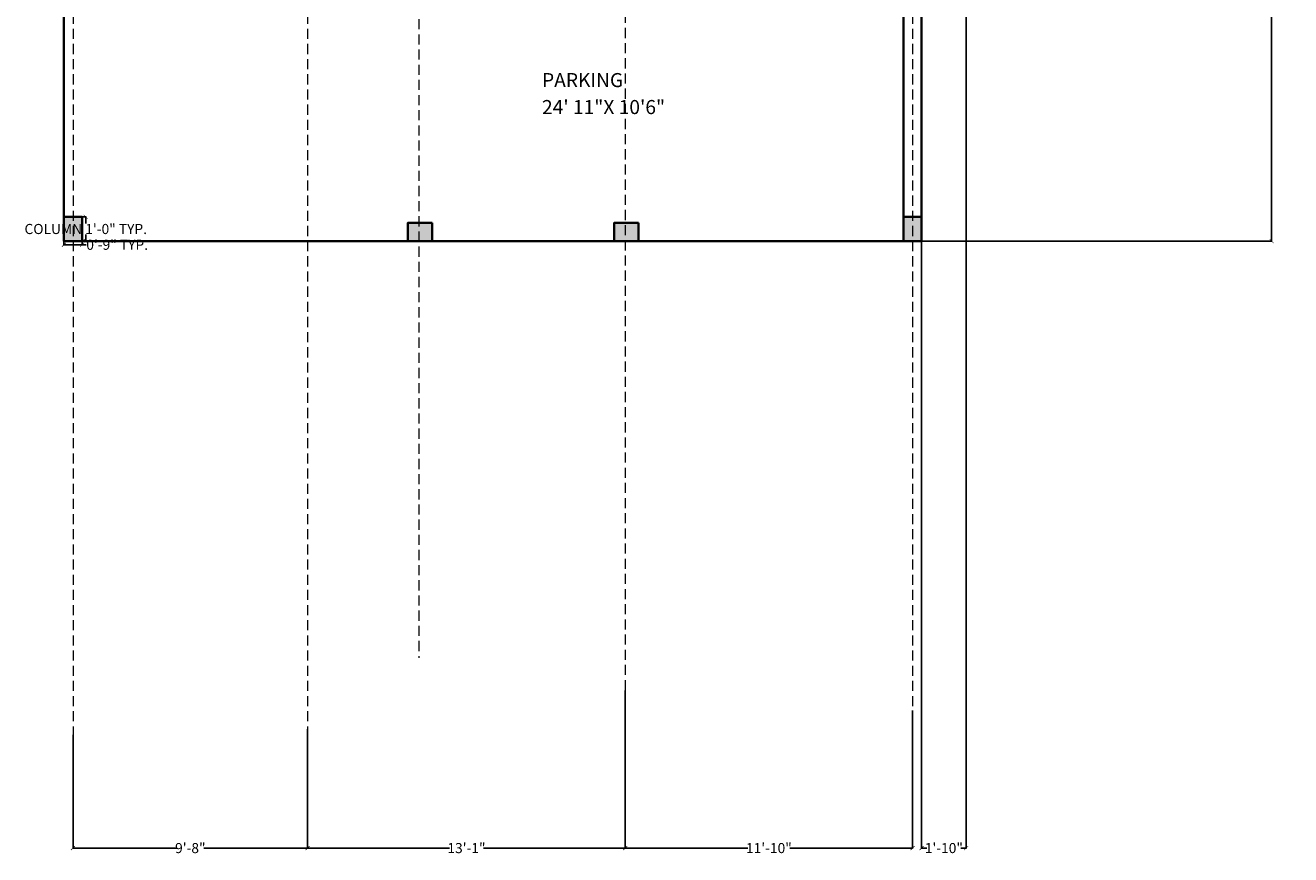
# Model space of a CAD drawing. Units: inches. Extents: x 782 to 2660, y -1008 to 166.
# Tile 1 of 12: x 964 to 1589, y -1008 to -598. Entities that reach past the tile are written whole.
import ezdxf

# ---------------------------------------------------------------- set-up
doc = ezdxf.new("R2010")
doc.units = ezdxf.units.IN
doc.header["$MEASUREMENT"] = 0
doc.linetypes.add('DASHED', pattern=[0.75, 0.5, -0.25])
for name, color, linetype, lineweight in [('A-ANNO-DIMS', 4, 'Continuous', 18), ('A-AREA-IDEN', 4, 'Continuous', 18), ('A-COLS', 7, 'Continuous', 35), ('A-GRID', 8, 'DASHED', 13), ('A-WALL', 7, 'Continuous', 35)]:
    doc.layers.add(name, color=color, linetype=linetype, lineweight=lineweight)
doc.styles.get("Standard").update_dxf_attribs({"font": 'arial.ttf'})
doc.dimstyles.get("Standard").update_dxf_attribs({"dimtxt": 5, "dimasz": 2, "dimexe": 0.18, "dimexo": 0.0625, "dimgap": 0.09, "dimtad": 0, "dimtih": 1, "dimtoh": 1, "dimdec": 0, "dimzin": 0, "dimdsep": 46, "dimlunit": 3, "dimtxsty": 'Standard', "dimblk": 'ARCHTICK', "dimcen": 0.09, "dimadec": 0, "dimazin": 0, "dimtfac": 1, "dimtdec": 0, "dimtofl": 0, "dimtmove": 0, "dimatfit": 3, "dimfxl": 1, "dimtolj": 1, "dimtzin": 0, "dimarcsym": 0})

# ---------------------------------------------------------------- blocks, each defined once
blk = doc.blocks.new('COL-9X12')
h = blk.add_hatch(color=256)
h.dxf.hatch_style = 1
h.paths.add_polyline_path([(9, 12), (0, 12), (0, 0), (9, 0)])
blk.add_lwpolyline([(0, 12), (9, 12), (9, 0), (0, 0)], close=True)
blk = doc.blocks.new('_ArchTick')
at = {"color": 0, "linetype": 'ByBlock', "const_width": 0.15}
blk.add_lwpolyline([(-0.5, -0.5), (0.5, 0.5)], dxfattribs=at)
blk = doc.blocks.new('*D25')
at = {"layer": 'A-ANNO-DIMS', "color": 0, "lineweight": -2, "transparency": 16777216}
for p, q in [((991.75, -692.99), (993.66, -692.99)), ((993.48, -692.99), (993.48, -696.32)), ((991.75, -704.99), (993.66, -704.99)), ((993.48, -704.99), (993.48, -701.67))]:
    blk.add_line(p, q, dxfattribs=at)
at = {"layer": 'Defpoints', "color": 0, "transparency": 16777216}
for p in [(991.68, -692.99), (993.48, -692.99), (991.68, -704.99)]:
    blk.add_point(p, dxfattribs=at)
at = {"layer": 'A-ANNO-DIMS', "color": 0, "lineweight": -2, "transparency": 16777216, "xscale": 2, "yscale": 2, "zscale": 2}
for p, rotation in [((993.48, -692.99), 90), ((993.48, -704.99), 270)]:
    blk.add_blockref('_ArchTick', p, dxfattribs=dict(at, rotation=rotation))
at = {"layer": 'A-ANNO-DIMS', "color": 0, "transparency": 16777216, "insert": (993.48, -698.99), "char_height": 5, "attachment_point": 5}
blk.add_mtext('\\A1;COLUMN 1\'-0" TYP.', dxfattribs=at)
blk = doc.blocks.new('*D26')
at = {"layer": 'A-ANNO-DIMS', "color": 0, "lineweight": -2, "transparency": 16777216}
for p, q in [((982.68, -705.06), (982.68, -706.97)), ((982.68, -706.79), (991.68, -706.79)), ((991.68, -705.06), (991.68, -706.97)), ((991.68, -706.79), (993.68, -706.79))]:
    blk.add_line(p, q, dxfattribs=at)
at = {"layer": 'Defpoints', "color": 0, "transparency": 16777216}
for p in [(982.68, -704.99), (991.68, -704.99), (991.68, -706.79)]:
    blk.add_point(p, dxfattribs=at)
at = {"layer": 'A-ANNO-DIMS', "color": 0, "lineweight": -2, "transparency": 16777216, "xscale": 2, "yscale": 2, "zscale": 2, "rotation": 180}
blk.add_blockref('_ArchTick', (982.68, -706.79), dxfattribs=at)
at = {"layer": 'A-ANNO-DIMS', "color": 0, "lineweight": -2, "transparency": 16777216, "xscale": 2, "yscale": 2, "zscale": 2}
blk.add_blockref('_ArchTick', (991.68, -706.79), dxfattribs=at)
at = {"layer": 'A-ANNO-DIMS', "color": 0, "transparency": 16777216, "insert": (1009.01, -706.79), "char_height": 5, "attachment_point": 5}
blk.add_mtext('\\A1;0\'-9" TYP.', dxfattribs=at)
blk = doc.blocks.new('*D51')
at = {"layer": 'A-ANNO-DIMS', "color": 0, "lineweight": -2, "transparency": 16777216}
for p, q in [((1406.75, 45.01), (1579.89, 45.01)), ((1579.71, 45.01), (1579.71, -327.35)), ((1579.71, -704.99), (1579.71, -332.64)), ((1406.75, -704.99), (1579.89, -704.99))]:
    blk.add_line(p, q, dxfattribs=at)
at = {"layer": 'Defpoints', "color": 0, "transparency": 16777216}
for p in [(1406.68, 45.01), (1579.71, 45.01), (1406.68, -704.99)]:
    blk.add_point(p, dxfattribs=at)
at = {"layer": 'A-ANNO-DIMS', "color": 0, "lineweight": -2, "transparency": 16777216, "xscale": 2, "yscale": 2, "zscale": 2}
for p, rotation in [((1579.71, 45.01), 90), ((1579.71, -704.99), 270)]:
    blk.add_blockref('_ArchTick', p, dxfattribs=dict(at, rotation=rotation))
at = {"layer": 'A-ANNO-DIMS', "color": 0, "transparency": 16777216, "insert": (1579.71, -329.99), "char_height": 5, "attachment_point": 5}
blk.add_mtext('\\A1;62\'-6"', dxfattribs=at)
blk = doc.blocks.new('*D53')
at = {"layer": 'A-ANNO-DIMS', "color": 0, "lineweight": -2, "transparency": 16777216}
for p, q in [((1406.68, -579.06), (1406.68, -1005.36)), ((1428.68, -579.06), (1428.68, -1005.36)), ((1406.68, -1005.18), (1409.24, -1005.18)), ((1428.68, -1005.18), (1426.13, -1005.18))]:
    blk.add_line(p, q, dxfattribs=at)
at = {"layer": 'Defpoints', "color": 0, "transparency": 16777216}
for p in [(1406.68, -578.99), (1428.68, -578.99), (1428.68, -1005.18)]:
    blk.add_point(p, dxfattribs=at)
at = {"layer": 'A-ANNO-DIMS', "color": 0, "lineweight": -2, "transparency": 16777216, "xscale": 2, "yscale": 2, "zscale": 2, "rotation": 180}
blk.add_blockref('_ArchTick', (1406.68, -1005.18), dxfattribs=at)
at = {"layer": 'A-ANNO-DIMS', "color": 0, "lineweight": -2, "transparency": 16777216, "xscale": 2, "yscale": 2, "zscale": 2}
blk.add_blockref('_ArchTick', (1428.68, -1005.18), dxfattribs=at)
at = {"layer": 'A-ANNO-DIMS', "color": 0, "transparency": 16777216, "insert": (1417.68, -1005.18), "char_height": 5, "attachment_point": 5}
blk.add_mtext('\\A1;1\'-10"', dxfattribs=at)
blk = doc.blocks.new('*D55')
at = {"layer": 'A-ANNO-DIMS', "color": 0, "lineweight": -2, "transparency": 16777216}
for p, q in [((987.18, -949.09), (987.18, -1005.36)), ((1103.18, -946.44), (1103.18, -1005.36)), ((987.18, -1005.18), (1038.45, -1005.18)), ((1103.18, -1005.18), (1051.92, -1005.18))]:
    blk.add_line(p, q, dxfattribs=at)
at = {"layer": 'Defpoints', "color": 0, "transparency": 16777216}
for p in [(987.18, -949.03), (1103.18, -946.37), (1103.18, -1005.18)]:
    blk.add_point(p, dxfattribs=at)
at = {"layer": 'A-ANNO-DIMS', "color": 0, "lineweight": -2, "transparency": 16777216, "xscale": 2, "yscale": 2, "zscale": 2, "rotation": 180}
blk.add_blockref('_ArchTick', (987.18, -1005.18), dxfattribs=at)
at = {"layer": 'A-ANNO-DIMS', "color": 0, "lineweight": -2, "transparency": 16777216, "xscale": 2, "yscale": 2, "zscale": 2}
blk.add_blockref('_ArchTick', (1103.18, -1005.18), dxfattribs=at)
at = {"layer": 'A-ANNO-DIMS', "color": 0, "transparency": 16777216, "insert": (1045.18, -1005.18), "char_height": 5, "attachment_point": 5}
blk.add_mtext('\\A1;9\'-8"', dxfattribs=at)
blk = doc.blocks.new('*D56')
at = {"layer": 'A-ANNO-DIMS', "color": 0, "lineweight": -2, "transparency": 16777216}
for p, q in [((1260.18, -927.18), (1260.18, -1005.36)), ((1103.18, -946.44), (1103.18, -1005.36)), ((1103.18, -1005.18), (1173.24, -1005.18)), ((1260.18, -1005.18), (1190.13, -1005.18))]:
    blk.add_line(p, q, dxfattribs=at)
at = {"layer": 'Defpoints', "color": 0, "transparency": 16777216}
for p in [(1260.18, -927.11), (1103.18, -946.37), (1260.18, -1005.18)]:
    blk.add_point(p, dxfattribs=at)
at = {"layer": 'A-ANNO-DIMS', "color": 0, "lineweight": -2, "transparency": 16777216, "xscale": 2, "yscale": 2, "zscale": 2, "rotation": 180}
blk.add_blockref('_ArchTick', (1103.18, -1005.18), dxfattribs=at)
at = {"layer": 'A-ANNO-DIMS', "color": 0, "lineweight": -2, "transparency": 16777216, "xscale": 2, "yscale": 2, "zscale": 2}
blk.add_blockref('_ArchTick', (1260.18, -1005.18), dxfattribs=at)
at = {"layer": 'A-ANNO-DIMS', "color": 0, "transparency": 16777216, "insert": (1181.68, -1005.18), "char_height": 5, "attachment_point": 5}
blk.add_mtext('\\A1;13\'-1"', dxfattribs=at)
blk = doc.blocks.new('*D57')
at = {"layer": 'A-ANNO-DIMS', "color": 0, "lineweight": -2, "transparency": 16777216}
for p, q in [((1260.18, -927.18), (1260.18, -1005.36)), ((1402.18, -937.2), (1402.18, -1005.36)), ((1260.18, -1005.18), (1320.8, -1005.18)), ((1402.18, -1005.18), (1341.57, -1005.18))]:
    blk.add_line(p, q, dxfattribs=at)
at = {"layer": 'Defpoints', "color": 0, "transparency": 16777216}
for p in [(1260.18, -927.11), (1402.18, -937.14), (1402.18, -1005.18)]:
    blk.add_point(p, dxfattribs=at)
at = {"layer": 'A-ANNO-DIMS', "color": 0, "lineweight": -2, "transparency": 16777216, "xscale": 2, "yscale": 2, "zscale": 2, "rotation": 180}
blk.add_blockref('_ArchTick', (1260.18, -1005.18), dxfattribs=at)
at = {"layer": 'A-ANNO-DIMS', "color": 0, "lineweight": -2, "transparency": 16777216, "xscale": 2, "yscale": 2, "zscale": 2}
blk.add_blockref('_ArchTick', (1402.18, -1005.18), dxfattribs=at)
at = {"layer": 'A-ANNO-DIMS', "color": 0, "transparency": 16777216, "insert": (1331.18, -1005.18), "char_height": 5, "attachment_point": 5}
blk.add_mtext('\\A1;11\'-10"', dxfattribs=at)

msp = doc.modelspace()

# ---------------------------------------------------------------- linework, layer by layer
at = {"layer": 'A-GRID', "ltscale": 10}
for p, q in [((987.18, 82.53), (987.18, -949.03)), ((1103.18, 82.53), (1103.18, -946.37)), ((1260.18, 82.94), (1260.18, -927.11)), ((1402.18, 82.53), (1402.18, -937.14)), ((1158.18, -340.22), (1158.18, -911.03))]:
    msp.add_line(p, q, dxfattribs=at)
at = {"layer": 'A-WALL'}
for p, q in [((982.68, 45.01), (982.68, -704.99)), ((1397.68, -578.99), (1397.68, -704.99)), ((1406.68, -704.99), (1406.68, -578.99)), ((1406.68, -704.99), (1406.68, -578.99)), ((1397.68, -704.99), (982.68, -704.99)), ((1397.68, -704.99), (1406.68, -704.99)), ((1397.68, -704.99), (1406.68, -704.99))]:
    msp.add_line(p, q, dxfattribs=at)

# ---------------------------------------------------------------- block references
at = {"layer": 'A-COLS'}
msp.add_blockref('COL-9X12', (982.68, -704.99), dxfattribs=at)
for p, rotation in [((1406.68, -692.99), 180), ((1152.67, -695.99), 270.0000000000002), ((1254.67, -695.99), 270.0000000000018)]:
    msp.add_blockref('COL-9X12', p, dxfattribs=dict(at, rotation=rotation))

# ---------------------------------------------------------------- texts
at = {"layer": 'A-AREA-IDEN'}
for s, height, p in [('PARKING', 6.958, (1219.03, -628.82)), ('24\' 11"X 10\'6"', 6.9576, (1219.03, -642.16))]:
    msp.add_text(s, height=height, dxfattribs=at).set_placement(p)

# ---------------------------------------------------------------- dimensions: what is measured, and where the dimension line sits
at = {"layer": 'A-ANNO-DIMS'}
dim = msp.add_linear_dim(base=(1579.71, 45.01), p1=(1406.68, -704.99), p2=(1406.68, 45.01), angle=90, dimstyle='Standard', override={"dimdec": 1, "dimlfac": 1, "dimrnd": 0, "dimzin": 1, "dimdsep": 46, "dimlunit": 4, "dimfrac": 2}, dxfattribs=at)
dim.commit()
dim.dimension.update_dxf_attribs({"geometry": '*D51', "text_midpoint": (1579.71, -329.99)})
for base, p1, p2, picture, middle in [((1428.68, -1005.18), (1406.68, -578.99), (1428.68, -578.99), '*D53', (1417.68, -1005.18)), ((1260.18, -1005.18), (1103.18, -946.37), (1260.18, -927.11), '*D56', (1181.68, -1005.18)), ((1402.18, -1005.18), (1260.18, -927.11), (1402.18, -937.14), '*D57', (1331.18, -1005.18)), ((1103.18, -1005.18), (987.18, -949.03), (1103.18, -946.37), '*D55', (1045.18, -1005.18))]:
    dim = msp.add_linear_dim(base=base, p1=p1, p2=p2, dimstyle='Standard', override={"dimdec": 1, "dimlfac": 1, "dimrnd": 0, "dimzin": 1, "dimdsep": 46, "dimlunit": 4, "dimfrac": 2}, dxfattribs=at)
    dim.commit()
    dim.dimension.update_dxf_attribs({"geometry": picture, "text_midpoint": middle})
dim = msp.add_linear_dim(base=(993.48, -692.99), p1=(991.68, -704.99), p2=(991.68, -692.99), angle=90, text='COLUMN <> TYP.', dimstyle='Standard', override={"dimdec": 1, "dimlfac": 1, "dimrnd": 0, "dimzin": 1, "dimdsep": 46, "dimlunit": 4, "dimfrac": 2}, dxfattribs=at)
dim.commit()
dim.dimension.update_dxf_attribs({"geometry": '*D25', "text_midpoint": (993.48, -698.99)})
dim = msp.add_linear_dim(base=(991.68, -706.79), p1=(982.68, -704.99), p2=(991.68, -704.99), text='<> TYP.', dimstyle='Standard', override={"dimdec": 1, "dimlfac": 1, "dimrnd": 0, "dimzin": 1, "dimdsep": 46, "dimlunit": 4, "dimfrac": 2}, dxfattribs=at)
dim.commit()
dim.dimension.update_dxf_attribs({"geometry": '*D26', "text_midpoint": (1009.01, -706.79)})

doc.saveas('drawing.dxf')
